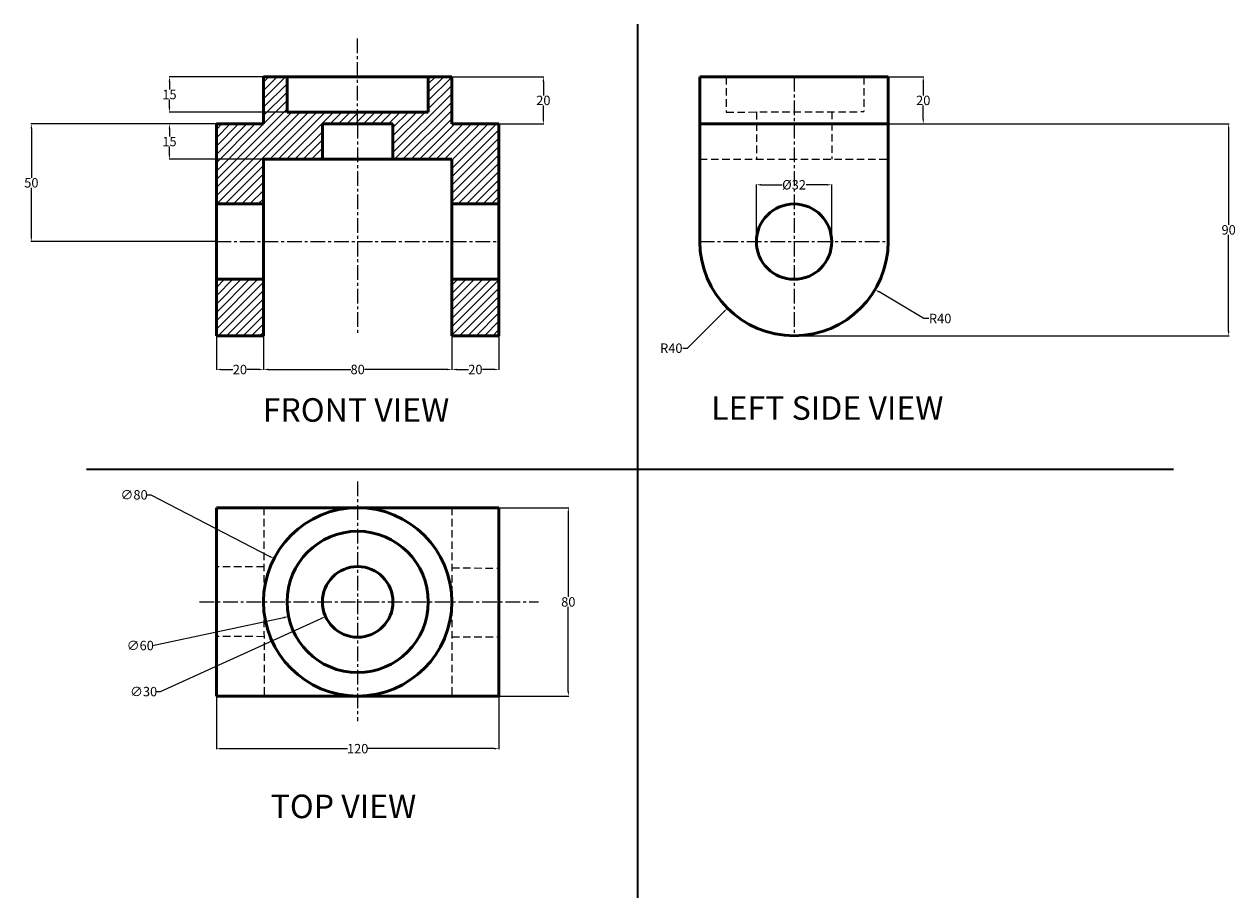
# Model space of a CAD drawing. Units: millimetres. Extents: x -475 to 40, y -900 to -205.
# Tile 1 of 1: x -474.8 to 39.6, y -900.5 to -529.4. Entities that reach past the tile are written whole.
import ezdxf

# ---------------------------------------------------------------- set-up
doc = ezdxf.new("R2010")
doc.units = ezdxf.units.MM
doc.header["$MEASUREMENT"] = 0
doc.linetypes.add('CENTER', pattern=[2, 1.25, -0.25, 0.25, -0.25])
doc.linetypes.add('HIDDEN', pattern=[9.524999999999999, 6.349999999999999, -3.174999999999999])
for name, color, linetype, lineweight in [('M-CNTR', 1, 'CENTER', 18), ('M-DIMS', 2, 'Continuous', 25), ('M-HATC', 8, 'Continuous', 18), ('M-HIDN', 3, 'HIDDEN', 25), ('M-OUTL', 7, 'Continuous', 50), ('M-TEXT', 7, 'Continuous', 25), ('M-TTLB', 7, 'Continuous', 35)]:
    doc.layers.add(name, color=color, linetype=linetype, lineweight=lineweight)
doc.styles.get("Standard").update_dxf_attribs({"font": 'arial.ttf'})
doc.dimstyles.get("Standard").update_dxf_attribs({"dimtxt": 4, "dimasz": 2, "dimexe": 0.18, "dimexo": 0.0625, "dimgap": 0.09, "dimtad": 0, "dimtih": 1, "dimtoh": 1, "dimdec": 0, "dimzin": 0, "dimdsep": 46, "dimtxsty": 'Standard', "dimcen": 0.09, "dimadec": 0, "dimazin": 0, "dimtfac": 1, "dimtdec": 0, "dimtofl": 0, "dimtmove": 0, "dimatfit": 3, "dimfxl": 1, "dimtolj": 1, "dimtzin": 0, "dimarcsym": 0})

# ---------------------------------------------------------------- blocks, each defined once
blk = doc.blocks.new('*D7')
at = {"layer": 'Defpoints', "color": 0, "transparency": 16777216}
for p in [(-393.2548938143664, -661.7501206102835), (-373.2548938143663, -661.7501206102835), (-373.2548938143663, -676.0556187403258)]:
    blk.add_point(p, dxfattribs=at)
at = {"layer": 'M-DIMS', "color": 0, "lineweight": -2, "transparency": 16777216}
for p, q in [((-393.2548938143664, -661.8126206102836), (-393.2548938143664, -676.2356187403257)), ((-373.2548938143663, -661.8126206102836), (-373.2548938143663, -676.2356187403257)), ((-391.2548938143664, -676.0556187403258), (-386.2371175524291, -676.0556187403258)), ((-375.2548938143663, -676.0556187403258), (-380.2726700763036, -676.0556187403258))]:
    blk.add_line(p, q, dxfattribs=at)
at = {"layer": 'M-DIMS', "color": 0, "transparency": 16777216}
for points in [[(-391.2548938143664, -675.7222854069925), (-391.2548938143664, -676.3889520736592), (-393.2548938143664, -676.0556187403258)], [(-375.2548938143663, -675.7222854069925), (-375.2548938143663, -676.3889520736592), (-373.2548938143663, -676.0556187403258)]]:
    blk.add_solid(points, dxfattribs=at)
at = {"layer": 'M-DIMS', "color": 0, "transparency": 16777216, "insert": (-383.2548938143664, -676.0556187403258), "char_height": 4, "attachment_point": 5}
blk.add_mtext('\\A1;20', dxfattribs=at)
blk = doc.blocks.new('*D8')
at = {"layer": 'Defpoints', "color": 0, "transparency": 16777216}
for p in [(-373.2548938143664, -661.7501206102835), (-293.2548938143664, -661.7501206102835), (-293.2548938143664, -676.0556187403258)]:
    blk.add_point(p, dxfattribs=at)
at = {"layer": 'M-DIMS', "color": 0, "lineweight": -2, "transparency": 16777216}
for p, q in [((-373.2548938143664, -661.8126206102836), (-373.2548938143664, -676.2356187403257)), ((-293.2548938143664, -661.8126206102836), (-293.2548938143664, -676.2356187403257)), ((-371.2548938143664, -676.0556187403258), (-336.2057396533841, -676.0556187403258)), ((-295.2548938143664, -676.0556187403258), (-330.3040479753486, -676.0556187403258))]:
    blk.add_line(p, q, dxfattribs=at)
at = {"layer": 'M-DIMS', "color": 0, "transparency": 16777216}
for points in [[(-371.2548938143664, -675.7222854069925), (-371.2548938143664, -676.3889520736592), (-373.2548938143664, -676.0556187403258)], [(-295.2548938143664, -675.7222854069925), (-295.2548938143664, -676.3889520736592), (-293.2548938143664, -676.0556187403258)]]:
    blk.add_solid(points, dxfattribs=at)
at = {"layer": 'M-DIMS', "color": 0, "transparency": 16777216, "insert": (-333.2548938143664, -676.0556187403258), "char_height": 4, "attachment_point": 5}
blk.add_mtext('\\A1;80', dxfattribs=at)
blk = doc.blocks.new('*D9')
at = {"layer": 'Defpoints', "color": 0, "transparency": 16777216}
for p in [(-293.2548938143664, -661.7501206102835), (-273.2548938143664, -661.7501206102835), (-273.2548938143664, -676.0556187403258)]:
    blk.add_point(p, dxfattribs=at)
at = {"layer": 'M-DIMS', "color": 0, "lineweight": -2, "transparency": 16777216}
for p, q in [((-293.2548938143664, -661.8126206102836), (-293.2548938143664, -676.2356187403257)), ((-273.2548938143664, -661.8126206102836), (-273.2548938143664, -676.2356187403257)), ((-291.2548938143664, -676.0556187403258), (-286.2371175524291, -676.0556187403258)), ((-275.2548938143664, -676.0556187403258), (-280.2726700763036, -676.0556187403258))]:
    blk.add_line(p, q, dxfattribs=at)
at = {"layer": 'M-DIMS', "color": 0, "transparency": 16777216}
for points in [[(-291.2548938143664, -675.7222854069925), (-291.2548938143664, -676.3889520736592), (-293.2548938143664, -676.0556187403258)], [(-275.2548938143664, -675.7222854069925), (-275.2548938143664, -676.3889520736592), (-273.2548938143664, -676.0556187403258)]]:
    blk.add_solid(points, dxfattribs=at)
at = {"layer": 'M-DIMS', "color": 0, "transparency": 16777216, "insert": (-283.2548938143664, -676.0556187403258), "char_height": 4, "attachment_point": 5}
blk.add_mtext('\\A1;20', dxfattribs=at)
blk = doc.blocks.new('*D10')
at = {"layer": 'Defpoints', "color": 0, "transparency": 16777216}
for p in [(-413.1784267098259, -571.7501206102837), (-373.2548938143664, -571.7501206102837), (-373.2548938143664, -586.7501206102836)]:
    blk.add_point(p, dxfattribs=at)
at = {"layer": 'M-DIMS', "color": 0, "lineweight": -2, "transparency": 16777216}
for p, q in [((-373.3173938143664, -571.7501206102837), (-413.3584267098259, -571.7501206102837)), ((-413.1784267098259, -573.7501206102836), (-413.1784267098259, -577.1178286593969)), ((-413.1784267098259, -584.7501206102837), (-413.1784267098259, -581.3824125611704)), ((-373.3173938143664, -586.7501206102836), (-413.3584267098259, -586.7501206102836))]:
    blk.add_line(p, q, dxfattribs=at)
at = {"layer": 'M-DIMS', "color": 0, "transparency": 16777216}
for points in [[(-413.5117600431593, -573.7501206102836), (-412.8450933764926, -573.7501206102836), (-413.1784267098259, -571.7501206102837)], [(-413.5117600431593, -584.7501206102837), (-412.8450933764926, -584.7501206102837), (-413.1784267098259, -586.7501206102836)]]:
    blk.add_solid(points, dxfattribs=at)
at = {"layer": 'M-DIMS', "color": 0, "transparency": 16777216, "insert": (-413.178426709826, -579.2501206102834), "char_height": 4, "attachment_point": 5}
blk.add_mtext('\\A1;15', dxfattribs=at)
blk = doc.blocks.new('*D11')
at = {"layer": 'Defpoints', "color": 0, "transparency": 16777216}
for p in [(-413.1784267098264, -551.7501206102838), (-363.2548938143665, -551.7501206102838), (-363.2548938143665, -566.7501206102838)]:
    blk.add_point(p, dxfattribs=at)
at = {"layer": 'M-DIMS', "color": 0, "lineweight": -2, "transparency": 16777216}
for p, q in [((-363.3173938143665, -551.7501206102838), (-413.3584267098264, -551.7501206102838)), ((-413.1784267098264, -553.7501206102838), (-413.1784267098264, -557.1178286593971)), ((-413.1784267098264, -564.7501206102838), (-413.1784267098264, -561.3824125611706)), ((-363.3173938143665, -566.7501206102838), (-413.3584267098264, -566.7501206102838))]:
    blk.add_line(p, q, dxfattribs=at)
at = {"layer": 'M-DIMS', "color": 0, "transparency": 16777216}
for points in [[(-413.5117600431597, -553.7501206102838), (-412.8450933764931, -553.7501206102838), (-413.1784267098264, -551.7501206102838)], [(-413.5117600431597, -564.7501206102838), (-412.8450933764931, -564.7501206102838), (-413.1784267098264, -566.7501206102838)]]:
    blk.add_solid(points, dxfattribs=at)
at = {"layer": 'M-DIMS', "color": 0, "transparency": 16777216, "insert": (-413.1784267098264, -559.2501206102836), "char_height": 4, "attachment_point": 5}
blk.add_mtext('\\A1;15', dxfattribs=at)
blk = doc.blocks.new('*D12')
at = {"layer": 'Defpoints', "color": 0, "transparency": 16777216}
for p in [(-293.2548938143665, -551.7501206102838), (-254.3879703025318, -551.7501206102837), (-293.2548938143665, -571.7501206102838)]:
    blk.add_point(p, dxfattribs=at)
at = {"layer": 'M-DIMS', "color": 0, "lineweight": -2, "transparency": 16777216}
for p, q in [((-293.1923938143665, -551.7501206102838), (-254.2079703025318, -551.7501206102837)), ((-254.3879703025318, -553.7501206102837), (-254.3879703025318, -559.6178286593969)), ((-254.3879703025318, -569.7501206102836), (-254.3879703025318, -563.8824125611704)), ((-293.1923938143665, -571.7501206102838), (-254.2079703025318, -571.7501206102837))]:
    blk.add_line(p, q, dxfattribs=at)
at = {"layer": 'M-DIMS', "color": 0, "transparency": 16777216}
for points in [[(-254.7213036358652, -553.7501206102837), (-254.0546369691984, -553.7501206102837), (-254.3879703025318, -551.7501206102837)], [(-254.7213036358652, -569.7501206102836), (-254.0546369691984, -569.7501206102836), (-254.3879703025318, -571.7501206102837)]]:
    blk.add_solid(points, dxfattribs=at)
at = {"layer": 'M-DIMS', "color": 0, "transparency": 16777216, "insert": (-254.3879703025319, -561.7501206102835), "char_height": 4, "attachment_point": 5}
blk.add_mtext('\\A1;20', dxfattribs=at)
blk = doc.blocks.new('*D13')
at = {"layer": 'Defpoints', "color": 0, "transparency": 16777216}
for p in [(-393.2548938143664, -814.7931227209474), (-273.2548938143664, -814.7931227209474), (-273.2548938143664, -837.1353569830425)]:
    blk.add_point(p, dxfattribs=at)
at = {"layer": 'M-DIMS', "color": 0, "lineweight": -2, "transparency": 16777216}
for p, q in [((-393.2548938143664, -814.8556227209473), (-393.2548938143664, -837.3153569830424)), ((-273.2548938143664, -814.8556227209473), (-273.2548938143664, -837.3153569830424)), ((-391.2548938143664, -837.1353569830425), (-337.5686318771222, -837.1353569830425)), ((-275.2548938143664, -837.1353569830425), (-328.9411557516106, -837.1353569830425))]:
    blk.add_line(p, q, dxfattribs=at)
at = {"layer": 'M-DIMS', "color": 0, "transparency": 16777216}
for points in [[(-391.2548938143664, -836.8020236497091), (-391.2548938143664, -837.468690316376), (-393.2548938143664, -837.1353569830425)], [(-275.2548938143664, -836.8020236497091), (-275.2548938143664, -837.468690316376), (-273.2548938143664, -837.1353569830425)]]:
    blk.add_solid(points, dxfattribs=at)
at = {"layer": 'M-DIMS', "color": 0, "transparency": 16777216, "insert": (-333.2548938143664, -837.1353569830425), "char_height": 4, "attachment_point": 5}
blk.add_mtext('\\A1;120', dxfattribs=at)
blk = doc.blocks.new('*D14')
at = {"layer": 'Defpoints', "color": 0, "transparency": 16777216}
for p in [(-273.2548938143665, -734.7931227209477), (-243.7951215102971, -734.7931227209476), (-273.2548938143665, -814.7931227209478)]:
    blk.add_point(p, dxfattribs=at)
at = {"layer": 'M-DIMS', "color": 0, "lineweight": -2, "transparency": 16777216}
for p, q in [((-273.1923938143665, -734.7931227209477), (-243.6151215102971, -734.7931227209476)), ((-243.7951215102971, -736.7931227209476), (-243.7951215102971, -772.660830770061)), ((-243.7951215102971, -812.7931227209478), (-243.7951215102971, -776.9254146718345)), ((-273.1923938143665, -814.7931227209478), (-243.6151215102971, -814.7931227209477))]:
    blk.add_line(p, q, dxfattribs=at)
at = {"layer": 'M-DIMS', "color": 0, "transparency": 16777216}
for points in [[(-244.1284548436305, -736.7931227209476), (-243.4617881769638, -736.7931227209476), (-243.7951215102971, -734.7931227209476)], [(-244.1284548436305, -812.7931227209478), (-243.4617881769638, -812.7931227209478), (-243.7951215102971, -814.7931227209477)]]:
    blk.add_solid(points, dxfattribs=at)
at = {"layer": 'M-DIMS', "color": 0, "transparency": 16777216, "insert": (-243.7951215102973, -774.7931227209475), "char_height": 4, "attachment_point": 5}
blk.add_mtext('\\A1;80', dxfattribs=at)
blk = doc.blocks.new('*D15')
at = {"layer": 'Defpoints', "color": 0, "transparency": 16777216}
for p in [(-319.6011326368391, -768.5822608075694), (-346.9086549918935, -781.0039846343254)]:
    blk.add_point(p, dxfattribs=at)
at = {"layer": 'M-DIMS', "color": 0, "lineweight": -2, "transparency": 16777216}
for p, q in [((-333.3448938143664, -774.7931227209473), (-333.1648938143664, -774.7931227209473)), ((-333.2548938143664, -774.8831227209475), (-333.2548938143663, -774.7031227209474)), ((-417.0176032462527, -812.8953434209928), (-348.7291564822306, -781.8320995561093)), ((-419.0176032462528, -812.8953434209928), (-417.0176032462527, -812.8953434209928))]:
    blk.add_line(p, q, dxfattribs=at)
at = {"layer": 'M-DIMS', "color": 0, "transparency": 16777216}
blk.add_solid([(-348.8671756358612, -781.528682641053), (-348.5911373285999, -782.1355164711653), (-346.9086549918935, -781.0039846343254)], dxfattribs=at)
at = {"layer": 'M-DIMS', "color": 0, "transparency": 16777216, "insert": (-424.1417096582583, -812.8953434209928), "char_height": 4, "attachment_point": 5}
blk.add_mtext('\\A1;∅30', dxfattribs=at)
blk = doc.blocks.new('*D16')
at = {"layer": 'Defpoints', "color": 0, "transparency": 16777216}
for p in [(-303.9099387727912, -768.5582519437831), (-362.5998488559412, -781.0279934981124)]:
    blk.add_point(p, dxfattribs=at)
at = {"layer": 'M-DIMS', "color": 0, "lineweight": -2, "transparency": 16777216}
for p, q in [((-333.3448938143662, -774.7931227209478), (-333.1648938143663, -774.7931227209478)), ((-333.2548938143663, -774.8831227209478), (-333.2548938143663, -774.7031227209478)), ((-420.4385157158482, -793.3168729080173), (-364.5561791920462, -781.4436515499234))]:
    blk.add_line(p, q, dxfattribs=at)
at = {"layer": 'M-DIMS', "color": 0, "transparency": 16777216}
blk.add_solid([(-364.6254555340147, -781.1175964939057), (-364.4869028500778, -781.7697066059409), (-362.5998488559412, -781.0279934981124)], dxfattribs=at)
at = {"layer": 'M-DIMS', "color": 0, "transparency": 16777216, "insert": (-425.5626221278538, -793.3168729080173), "char_height": 4, "attachment_point": 5}
blk.add_mtext('\\A1;∅60', dxfattribs=at)
blk = doc.blocks.new('*D17')
at = {"layer": 'Defpoints', "color": 0, "transparency": 16777216}
for p in [(-368.7707073056375, -756.391302374763), (-297.7390803230952, -793.1949430671317)]:
    blk.add_point(p, dxfattribs=at)
at = {"layer": 'M-DIMS', "color": 0, "lineweight": -2, "transparency": 16777216}
for p, q in [((-423.0604957758403, -729.2983767515013), (-421.0604957758397, -729.2983767515013)), ((-421.0604957758397, -729.2983767515013), (-370.546497980201, -755.4712113574539)), ((-333.3448938143662, -774.7931227209473), (-333.1648938143664, -774.7931227209475)), ((-333.2548938143663, -774.8831227209475), (-333.2548938143663, -774.7031227209474))]:
    blk.add_line(p, q, dxfattribs=at)
at = {"layer": 'M-DIMS', "color": 0, "transparency": 16777216}
blk.add_solid([(-370.3931494773161, -755.1752462450265), (-370.6998464830859, -755.7671764698811), (-368.7707073056375, -756.391302374763)], dxfattribs=at)
at = {"layer": 'M-DIMS', "color": 0, "transparency": 16777216, "insert": (-428.1846021878457, -729.2983767515013), "char_height": 4, "attachment_point": 5}
blk.add_mtext('\\A1;∅80', dxfattribs=at)
blk = doc.blocks.new('*D18')
at = {"layer": 'Defpoints', "color": 0, "transparency": 16777216}
for p in [(-107.9421157920961, -551.7501206102838), (-107.9421157920961, -571.750120610284), (-93.06794504656693, -571.750120610284)]:
    blk.add_point(p, dxfattribs=at)
at = {"layer": 'M-DIMS', "color": 0, "lineweight": -2, "transparency": 16777216}
for p, q in [((-107.8796157920961, -551.7501206102838), (-92.88794504656693, -551.7501206102838)), ((-93.06794504656693, -553.7501206102838), (-93.06794504656693, -559.6178286593972)), ((-93.06794504656693, -569.750120610284), (-93.06794504656693, -563.8824125611706)), ((-107.8796157920961, -571.750120610284), (-92.88794504656693, -571.750120610284))]:
    blk.add_line(p, q, dxfattribs=at)
at = {"layer": 'M-DIMS', "color": 0, "transparency": 16777216}
for points in [[(-93.40127837990026, -553.7501206102838), (-92.7346117132336, -553.7501206102838), (-93.06794504656693, -551.7501206102838)], [(-93.40127837990026, -569.750120610284), (-92.7346117132336, -569.750120610284), (-93.06794504656693, -571.750120610284)]]:
    blk.add_solid(points, dxfattribs=at)
at = {"layer": 'M-DIMS', "color": 0, "transparency": 16777216, "insert": (-93.06794504656708, -561.7501206102838), "char_height": 4, "attachment_point": 5}
blk.add_mtext('\\A1;20', dxfattribs=at)
blk = doc.blocks.new('*D19')
at = {"layer": 'Defpoints', "color": 0, "transparency": 16777216}
for p in [(-147.942115792096, -621.7501206102834), (-113.5130013151839, -642.1127352836421)]:
    blk.add_point(p, dxfattribs=at)
at = {"layer": 'M-DIMS', "color": 0, "lineweight": -2, "transparency": 16777216}
for p, q in [((-148.032115792096, -621.7501206102834), (-147.8521157920959, -621.7501206102836)), ((-147.942115792096, -621.8401206102836), (-147.9421157920961, -621.6601206102835)), ((-92.75200127145486, -654.391536250409), (-111.7915455913383, -643.13086601731)), ((-90.75200127145487, -654.391536250409), (-92.75200127145486, -654.391536250409))]:
    blk.add_line(p, q, dxfattribs=at)
at = {"layer": 'M-DIMS', "color": 0, "transparency": 16777216}
blk.add_solid([(-111.621857135727, -642.8439567300024), (-111.9612340469496, -643.4177753046176), (-113.5130013151839, -642.1127352836421)], dxfattribs=at)
at = {"layer": 'M-DIMS', "color": 0, "transparency": 16777216, "insert": (-85.88983210365134, -654.391536250409), "char_height": 4, "attachment_point": 5}
blk.add_mtext('\\A1;R40', dxfattribs=at)
blk = doc.blocks.new('*D20')
at = {"layer": 'Defpoints', "color": 0, "transparency": 16777216}
for p in [(-131.942115792096, -597.5989959539078), (-163.942115792096, -621.7501206102836), (-131.942115792096, -621.7501206102836)]:
    blk.add_point(p, dxfattribs=at)
at = {"layer": 'M-DIMS', "color": 0, "lineweight": -2, "transparency": 16777216}
for p, q in [((-163.942115792096, -621.6876206102836), (-163.942115792096, -597.4189959539079)), ((-161.942115792096, -597.5989959539078), (-153.0525796392993, -597.5989959539078)), ((-133.942115792096, -597.5989959539078), (-142.8316519448928, -597.5989959539078)), ((-131.942115792096, -621.6876206102836), (-131.942115792096, -597.4189959539079))]:
    blk.add_line(p, q, dxfattribs=at)
at = {"layer": 'M-DIMS', "color": 0, "transparency": 16777216}
for points in [[(-161.942115792096, -597.2656626205745), (-161.942115792096, -597.9323292872411), (-163.942115792096, -597.5989959539078)], [(-133.942115792096, -597.2656626205745), (-133.942115792096, -597.9323292872411), (-131.942115792096, -597.5989959539078)]]:
    blk.add_solid(points, dxfattribs=at)
at = {"layer": 'M-DIMS', "color": 0, "transparency": 16777216, "insert": (-147.942115792096, -597.5989959539078), "char_height": 4, "attachment_point": 5}
blk.add_mtext('\\A1;%%C32', dxfattribs=at)
blk = doc.blocks.new('*D21')
at = {"layer": 'Defpoints', "color": 0, "transparency": 16777216}
for p in [(-393.2548940000002, -571.7501210000001), (-471.8190230000004, -621.7501210000001), (-393.2548940000002, -621.7501210000001)]:
    blk.add_point(p, dxfattribs=at)
at = {"layer": 'M-DIMS', "color": 0, "lineweight": -2, "transparency": 16777216}
for p, q in [((-393.3173940000002, -571.7501210000001), (-471.9990230000004, -571.7501210000001)), ((-471.8190230000004, -573.7501210000003), (-471.8190230000004, -594.6178290491135)), ((-471.8190230000004, -619.7501210000003), (-471.8190230000004, -598.882412950887)), ((-393.3173940000002, -621.7501210000001), (-471.9990230000004, -621.7501210000001))]:
    blk.add_line(p, q, dxfattribs=at)
at = {"layer": 'M-DIMS', "color": 0, "transparency": 16777216}
for points in [[(-472.1523563333337, -573.7501210000003), (-471.4856896666671, -573.7501210000003), (-471.8190230000004, -571.7501210000001)], [(-472.1523563333337, -619.7501210000003), (-471.4856896666671, -619.7501210000003), (-471.8190230000004, -621.7501210000001)]]:
    blk.add_solid(points, dxfattribs=at)
at = {"layer": 'M-DIMS', "color": 0, "transparency": 16777216, "insert": (-471.8190230000005, -596.750121), "char_height": 4, "attachment_point": 5}
blk.add_mtext('\\A1;50', dxfattribs=at)
blk = doc.blocks.new('*D22')
at = {"layer": 'Defpoints', "color": 0, "transparency": 16777216}
for p in [(-107.942116, -571.7501210000001), (-147.942116, -661.7501210000003), (36.61534800000004, -661.7501210000003)]:
    blk.add_point(p, dxfattribs=at)
at = {"layer": 'M-DIMS', "color": 0, "lineweight": -2, "transparency": 16777216}
for p, q in [((-107.879616, -571.7501210000001), (36.79534800000002, -571.7501210000001)), ((36.61534800000002, -573.7501210000003), (36.61534800000003, -614.6178290491135)), ((36.61534800000004, -659.7501210000001), (36.61534800000003, -618.8824129508869)), ((-147.879616, -661.7501210000003), (36.79534800000003, -661.7501210000003))]:
    blk.add_line(p, q, dxfattribs=at)
at = {"layer": 'M-DIMS', "color": 0, "transparency": 16777216}
for points in [[(36.28201466666669, -573.7501210000003), (36.94868133333335, -573.7501210000003), (36.61534800000002, -571.7501210000001)], [(36.2820146666667, -659.7501210000001), (36.94868133333338, -659.7501210000001), (36.61534800000004, -661.7501210000003)]]:
    blk.add_solid(points, dxfattribs=at)
at = {"layer": 'M-DIMS', "color": 0, "transparency": 16777216, "insert": (36.61534799999985, -616.7501210000001), "char_height": 4, "attachment_point": 5}
blk.add_mtext('\\A1;90', dxfattribs=at)
blk = doc.blocks.new('*D23')
at = {"layer": 'Defpoints', "color": 0, "transparency": 16777216}
for p in [(-147.942116, -621.750121), (-176.225389, -650.03539)]:
    blk.add_point(p, dxfattribs=at)
at = {"layer": 'M-DIMS', "color": 0, "lineweight": -2, "transparency": 16777216}
for p, q in [((-148.032116, -621.750121), (-147.852116, -621.750121)), ((-147.942116, -621.840121), (-147.942116, -621.660121)), ((-193.1953529379081, -667.0065515379177), (-177.6395526614923, -651.4496534614932)), ((-195.195352937908, -667.0065515379177), (-193.1953529379081, -667.0065515379177))]:
    blk.add_line(p, q, dxfattribs=at)
at = {"layer": 'M-DIMS', "color": 0, "transparency": 16777216}
blk.add_solid([(-177.8752632384078, -651.2139595179111), (-177.4038420845768, -651.685347405075), (-176.225389, -650.03539)], dxfattribs=at)
at = {"layer": 'M-DIMS', "color": 0, "transparency": 16777216, "insert": (-200.0575221057117, -667.0065515379177), "char_height": 4, "attachment_point": 5}
blk.add_mtext('\\A1;R40', dxfattribs=at)

msp = doc.modelspace()

# ---------------------------------------------------------------- hatches: boundary and pattern name
at = {"layer": 'M-HATC'}
h = msp.add_hatch(dxfattribs=at)
h.set_pattern_fill('ANSI31', color=256, scale=20)
h.set_pattern_definition([(45, (-814.1415897467771, -347.9535343046347), (-1.767766952966368, 1.767766952966368), [])])
h.paths.add_polyline_path([(-373.2548938143663, -586.7501206102835), (-348.2548938143663, -586.7501206102835), (-348.2548938143663, -571.7501206102834), (-333.2548938143663, -571.7501206102836), (-333.2548938143663, -566.7501206102835), (-363.2548938143664, -566.7501206102835), (-363.2548938143664, -551.7501206102836), (-373.2548938143663, -551.7501206102836), (-373.2548938143663, -571.7501206102834), (-393.2548938143664, -571.7501206102836), (-393.2548938143664, -605.7501206102836), (-373.2548938143663, -605.7501206102834)])
h.paths.add_polyline_path([(-273.2548938143664, -571.7501206102836), (-293.2548938143664, -571.7501206102836), (-293.2548938143664, -551.7501206102836), (-303.2548938143663, -551.7501206102836), (-303.2548938143663, -566.7501206102835), (-333.2548938143663, -566.7501206102835), (-333.2548938143663, -571.7501206102836), (-318.2548938143662, -571.7501206102836), (-318.2548938143662, -586.7501206102835), (-293.2548938143664, -586.7501206102835), (-293.2548938143664, -605.7501206102836), (-273.2548938143664, -605.7501206102836)])
h.paths.add_polyline_path([(-273.2548938143664, -637.7501206102835), (-293.2548938143664, -637.7501206102834), (-293.2548938143664, -661.7501206102835), (-273.2548938143664, -661.7501206102835)])
h.paths.add_polyline_path([(-373.2548938143664, -637.7501206102834), (-393.2548938143664, -637.7501206102835), (-393.2548938143664, -661.7501206102835), (-373.2548938143664, -661.7501206102835)])

# ---------------------------------------------------------------- linework, layer by layer
at = {"layer": 'M-CNTR', "ltscale": 5}
for p, q in [((-333.2548938143663, -551.7501206102836), (-333.2548938143663, -535.4353280553617)), ((-333.2548938143663, -571.7501206102836), (-333.2548938143663, -551.7501206102836)), ((-147.942115792096, -551.7501206102836), (-147.942115792096, -661.7501206102835)), ((-333.2548938143663, -571.7501206102836), (-333.2548938143664, -661.7501206102835)), ((-393.2548938143664, -621.7501206102836), (-373.2548938143663, -621.7501206102834)), ((-373.2548938143663, -621.7501206102833), (-273.2548938143664, -621.7501206102836)), ((-187.942115792096, -621.7501206102836), (-107.942115792096, -621.7501206102837)), ((-333.2548938143663, -723.6895916259531), (-333.2548938143663, -825.4364704060067)), ((-400.4310808693926, -774.7931227209473), (-256.3934252059016, -774.7931227209473))]:
    msp.add_line(p, q, dxfattribs=at)
at = {"layer": 'M-HIDN', "ltscale": 0.5}
for p, q in [((-176.7454171463723, -551.7501206102837), (-176.7454171463723, -566.7141960062577)), ((-118.3706855688359, -551.7501206102836), (-118.3706855688359, -566.5269006986503)), ((-176.7454171463723, -566.7141960062577), (-118.3706855688359, -566.5269006986504)), ((-163.942115792096, -566.6699081182746), (-163.942115792096, -586.7501206102835)), ((-131.942115792096, -566.5736531278632), (-131.942115792096, -586.750120610283)), ((-187.942115792096, -586.7501206102835), (-107.942115792096, -586.7501206102836)), ((-373.1250074456879, -734.7931227209474), (-372.9827500193224, -814.7931227209474)), ((-293.2472788457413, -734.7931227209474), (-293.2389385876413, -814.7931227209474)), ((-373.0804185029707, -759.8681961882406), (-393.2548938143664, -759.9062262662947)), ((-293.2446246092811, -760.2526365961933), (-273.2548938143664, -760.4818394008657)), ((-373.0276047926465, -789.5685565411416), (-393.2548938143665, -789.4543484594769)), ((-293.2415551792725, -789.6946991484047), (-273.2548938143664, -789.646219504334))]:
    msp.add_line(p, q, dxfattribs=at)
at = {"layer": 'M-OUTL'}
for p, q in [((-373.2548938143663, -571.7501206102836), (-373.2548938143663, -551.7501206102836)), ((-373.2548938143663, -571.7501206102836), (-373.2548938143663, -551.7501206102836)), ((-373.2548938143663, -551.7501206102836), (-293.2548938143664, -551.7501206102836)), ((-363.2548938143664, -566.7501206102834), (-363.2548938143664, -551.7501206102836)), ((-363.2548938143664, -551.7501206102836), (-363.2548938143664, -566.7501206102835)), ((-303.2548938143663, -566.7501206102834), (-303.2548938143663, -551.7501206102836)), ((-293.2548938143664, -571.7501206102836), (-293.2548938143664, -551.7501206102836)), ((-187.942115792096, -551.7501206102837), (-107.942115792096, -551.7501206102836)), ((-187.942115792096, -551.7501206102837), (-187.942115792096, -621.7501206102836)), ((-187.942115792096, -551.7501206102837), (-107.942115792096, -551.7501206102837)), ((-107.942115792096, -551.7501206102837), (-107.942115792096, -621.7501206102837)), ((-363.2548938143664, -566.7501206102835), (-303.2548938143664, -566.7501206102835)), ((-393.2548938143664, -571.7501206102836), (-393.2548938143664, -661.7501206102835)), ((-373.2548938143663, -571.7501206102834), (-393.2548938143664, -571.7501206102836)), ((-348.2548938143663, -586.7501206102835), (-348.2548938143663, -571.7501206102836)), ((-318.2548938143662, -571.7501206102836), (-348.2548938143663, -571.7501206102834)), ((-318.2548938143662, -586.7501206102835), (-318.2548938143662, -571.7501206102836)), ((-273.2548938143664, -571.7501206102836), (-293.2548938143664, -571.7501206102836)), ((-273.2548938143664, -661.7501206102835), (-273.2548938143664, -571.7501206102836)), ((-187.942115792096, -571.7501206102837), (-107.942115792096, -571.7501206102837)), ((-373.2548938143663, -586.7501206102835), (-373.2548938143664, -661.7501206102835)), ((-293.2548938143663, -586.7501206102835), (-373.2548938143663, -586.7501206102835)), ((-293.2548938143664, -586.7501206102836), (-293.2548938143664, -661.7501206102835)), ((-393.2548938143664, -605.7501206102836), (-373.2548938143663, -605.7501206102834)), ((-293.2548938143664, -605.7501206102836), (-273.2548938143664, -605.7501206102836)), ((-393.2548938143664, -637.7501206102835), (-373.2548938143663, -637.7501206102834)), ((-293.2548938143664, -637.7501206102834), (-273.2548938143664, -637.7501206102835)), ((-393.2548938143664, -661.7501206102835), (-373.2548938143663, -661.7501206102835)), ((-293.2548938143664, -661.7501206102835), (-273.2548938143664, -661.7501206102835)), ((-393.2548938143664, -734.7931227209475), (-393.2548938143664, -814.7931227209474)), ((-393.2548938143664, -734.7931227209474), (-273.2548938143664, -734.7931227209475)), ((-393.2548938143664, -734.7931227209474), (-393.2548938143664, -814.7931227209474)), ((-273.2548938143664, -734.7931227209474), (-273.2548938143664, -814.7931227209474)), ((-273.2548938143664, -814.7931227209474), (-273.2548938143664, -734.7931227209474)), ((-333.2548938143663, -759.7931227209474), (-333.3114453860793, -759.7932293240017)), ((-333.3114453860371, -759.7932293240013), (-332.854423944339, -759.798469544458)), ((-333.4242755452195, -789.7921663514344), (-333.0127511468757, -789.7911681578895)), ((-333.2548938143663, -789.7931227209474), (-333.4242755452085, -789.7921663514344)), ((-393.2548938143664, -814.7931227209474), (-273.2548938143664, -814.7931227209474))]:
    msp.add_line(p, q, dxfattribs=at)
for centre, radius in [((-147.942115792096, -621.7501206102836), 16), ((-333.2548938143663, -774.7931227209473), 40), ((-333.2548938143663, -774.7931227209473), 30), ((-333.2548938143663, -774.7931227209473), 15)]:
    msp.add_circle(centre, radius, dxfattribs=at)
msp.add_arc((-147.942115792096, -621.7501206102836), 40, 180, 359.9999999999998, dxfattribs=at)
at = {"layer": 'M-TTLB'}
for p, q in [((-214.3663663864145, -529.3863867000968), (-214.3663663864145, -900.4814868801723)), ((-448.4190226990822, -718.466792025567), (13.21534828622134, -718.466792025567))]:
    msp.add_line(p, q, dxfattribs=at)

# ---------------------------------------------------------------- texts
at = {"layer": 'M-TEXT'}
for s, p in [('FRONT VIEW', (-373.6011047127758, -698.2561499433709)), ('LEFT SIDE VIEW', (-183.1410567236498, -697.429407166402)), ('TOP VIEW', (-370.2040809179525, -866.6550578738631))]:
    msp.add_text(s, height=10, dxfattribs=at).set_placement(p)

# ---------------------------------------------------------------- dimensions: what is measured, and where the dimension line sits
at = {"layer": 'M-DIMS'}
for base, p1, p2, override, picture, middle in [((-413.1784267098264, -551.7501206102838), (-363.2548938143664, -566.7501206102835), (-363.2548938143664, -551.7501206102836), {"dimclrd": 0, "dimclre": 0, "dimclrt": 0}, '*D11', (-413.1784267098264, -559.2501206102836)), ((-254.3879703025318, -551.7501206102837), (-293.2548938143664, -571.7501206102836), (-293.2548938143664, -551.7501206102836), {"dimclrd": 0, "dimclre": 0, "dimclrt": 0}, '*D12', (-254.3879703025319, -561.7501206102835)), ((-93.06794504656693, -571.750120610284), (-107.942115792096, -551.7501206102836), (-107.942115792096, -571.7501206102837), {"dimclrd": 0, "dimclre": 0, "dimclrt": 0}, '*D18', (-93.06794504656708, -561.7501206102838)), ((-471.8190230000004, -621.7501210000001), (-393.254894, -571.750121), (-393.254894, -621.750121), {"dimdec": 0, "dimlfac": 1, "dimrnd": 0, "dimzin": 0, "dimdsep": 46, "dimlunit": 2}, '*D21', (-471.8190230000005, -596.750121)), ((-413.1784267098259, -571.7501206102837), (-373.2548938143663, -586.7501206102835), (-373.2548938143663, -571.7501206102834), {"dimclrd": 0, "dimclre": 0, "dimclrt": 0}, '*D10', (-413.178426709826, -579.2501206102834)), ((36.61534800000004, -661.7501210000003), (-107.942116, -571.750121), (-147.942116, -661.750121), {"dimdec": 0, "dimlfac": 1, "dimrnd": 0, "dimzin": 0, "dimdsep": 46, "dimlunit": 2}, '*D22', (36.61534799999985, -616.7501210000001)), ((-243.7951215102971, -734.7931227209476), (-273.2548938143664, -814.7931227209474), (-273.2548938143664, -734.7931227209475), {"dimclrd": 0, "dimclre": 0, "dimclrt": 0}, '*D14', (-243.7951215102973, -774.7931227209475))]:
    dim = msp.add_linear_dim(base=base, p1=p1, p2=p2, angle=90, dimstyle='Standard', override=override, dxfattribs=at)
    dim.commit()
    dim.dimension.update_dxf_attribs({"geometry": picture, "text_midpoint": middle})
dim = msp.add_linear_dim(base=(-131.942115792096, -597.5989959539078), p1=(-163.942115792096, -621.7501206102836), p2=(-131.942115792096, -621.7501206102836), text='%%C<>', dimstyle='Standard', override={"dimclrd": 0, "dimclre": 0, "dimclrt": 0}, dxfattribs=at)
dim.commit()
dim.dimension.update_dxf_attribs({"geometry": '*D20', "text_midpoint": (-147.942115792096, -597.5989959539078)})
for center, mpoint, override, picture, middle in [((-147.942116, -621.750121), (-176.225389, -650.03539), {"dimdec": 0, "dimlfac": 1, "dimrnd": 0, "dimzin": 0, "dimdsep": 46, "dimlunit": 2}, '*D23', (-200.0575221057117, -667.0065515379177)), ((-147.942115792096, -621.7501206102834), (-113.5130013151839, -642.1127352836421), {"dimclrd": 0, "dimclre": 0, "dimclrt": 0}, '*D19', (-85.88983210365134, -654.391536250409))]:
    dim = msp.add_radius_dim(center=center, mpoint=mpoint, dimstyle='Standard', override=override, dxfattribs=at)
    dim.commit()
    dim.dimension.update_dxf_attribs({"geometry": picture, "text_midpoint": middle, "dimtype": 164})
for base, p1, p2, picture, middle in [((-373.2548938143663, -676.0556187403258), (-393.2548938143664, -661.7501206102835), (-373.2548938143663, -661.7501206102835), '*D7', (-383.2548938143664, -676.0556187403258)), ((-293.2548938143664, -676.0556187403258), (-373.2548938143664, -661.7501206102835), (-293.2548938143664, -661.7501206102835), '*D8', (-333.2548938143664, -676.0556187403258)), ((-273.2548938143664, -676.0556187403258), (-293.2548938143664, -661.7501206102835), (-273.2548938143664, -661.7501206102835), '*D9', (-283.2548938143664, -676.0556187403258)), ((-273.2548938143664, -837.1353569830425), (-393.2548938143664, -814.7931227209474), (-273.2548938143664, -814.7931227209474), '*D13', (-333.2548938143664, -837.1353569830425))]:
    dim = msp.add_linear_dim(base=base, p1=p1, p2=p2, dimstyle='Standard', override={"dimclrd": 0, "dimclre": 0, "dimclrt": 0}, dxfattribs=at)
    dim.commit()
    dim.dimension.update_dxf_attribs({"geometry": picture, "text_midpoint": middle})
for p1, p2, picture, middle in [((-297.7390803230952, -793.1949430671317), (-368.7707073056375, -756.391302374763), '*D17', (-428.1846021878457, -729.2983767515013)), ((-303.9099387727912, -768.5582519437831), (-362.5998488559412, -781.0279934981124), '*D16', (-420.4385157158482, -793.3168729080173)), ((-319.6011326368391, -768.5822608075694), (-346.9086549918935, -781.0039846343254), '*D15', (-424.1417096582583, -812.8953434209928))]:
    dim = msp.add_diameter_dim_2p(p1=p1, p2=p2, dimstyle='Standard', override={"dimclrd": 0, "dimclre": 0, "dimclrt": 0}, dxfattribs=at)
    dim.commit()
    dim.dimension.update_dxf_attribs({"geometry": picture, "text_midpoint": middle, "dimtype": 163})

doc.saveas('drawing.dxf')
